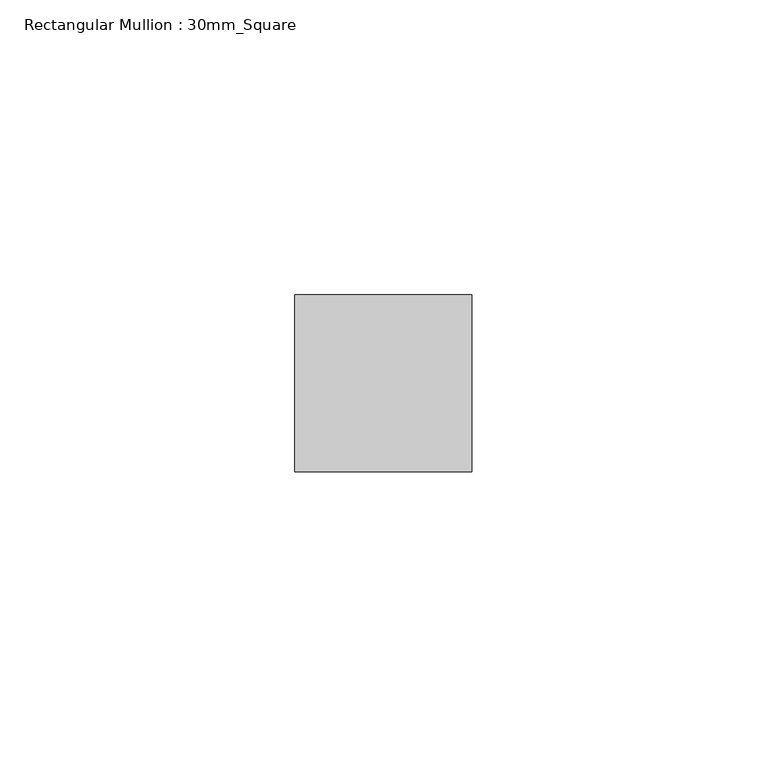
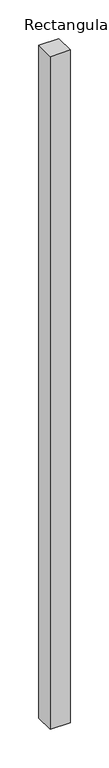
"""IFC4 building model written with IfcOpenShell, lengths in millimetres: member geometry, Rectangular Mullion : 30mm_Square."""

from ifc_helpers import new_model, si_unit, frame, origin, place, context, project, spatial, polyline, outline, extrude, source, transform, mapped, element, save


def rectangular_mullion_30mm_square_f98953c9(model_context):
    return source(origin(), model_context, "Body", "SweptSolid", [
        extrude(outline(polyline([(0.0, 15.0), (0.0, -15.0), (-30.0, -15.0), (-30.0, 15.0), (0.0, 15.0)])), frame((0.0, 0.0, -1066.8), z_axis=(0.0, 0.0, 1.0), x_axis=(1.0, 0.0, 0.0)), (0.0, 0.0, 1.0), 1066.8),
    ])


if __name__ == "__main__":
    model = new_model("IFC4")
    model_context = context("Model", 3, world=origin())
    ifc_project = project(units=[si_unit("LENGTHUNIT", "METRE", prefix="MILLI")], contexts=[model_context])
    site = spatial("IfcSite", under=ifc_project)
    building = spatial("IfcBuilding", under=site)
    placement = place(None, origin())
    rectangular_mullion_30mm_square_shape = rectangular_mullion_30mm_square_f98953c9(model_context)
    element("IfcMember", 1, ObjectType="Rectangular Mullion : 30mm_Square", at=placement, inside=building, context=model_context, shape_type="MappedRepresentation", body=[
        mapped(rectangular_mullion_30mm_square_shape, transform((0.0, 0.0, 0.0), x_axis=(1.0, 0.0, 0.0), y_axis=(0.0, 1.0, 0.0), z_axis=(0.0, 0.0, 1.0))),
    ])
    save(model, "model.ifc")

# Revit data of these elements
# Type "Rectangular Mullion : 30mm_Square"
#   Keynote = "H11"
#   built-in parameter 1007304 = 0.0984252 (stored number, unit not read)
#   built-in parameter 1007301 = 0.0492126 (stored number, unit not read)
#   built-in parameter 1007300 = 0.0492126 (stored number, unit not read)
# Element 1 (IfcMember, "Rectangular Mullion : 30mm_Square")
#   Materials on its faces: "Aluminium"
# Materials
#   "Aluminium": class "Metal", colour RGB 247 247 247, transparency 0, Description = "Aluminium 6061", Cost = 0
